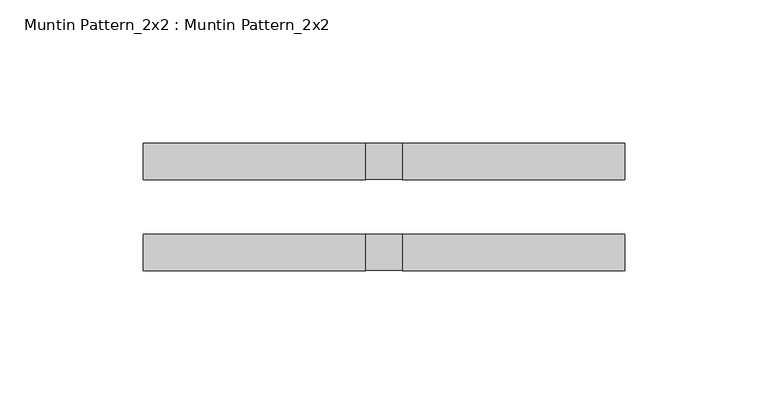
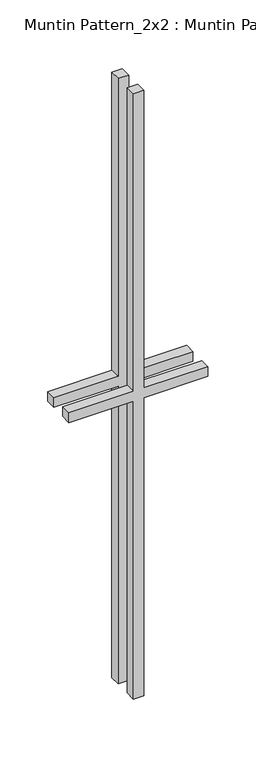
"""IFC4 building model written with IfcOpenShell, lengths in millimetres: proxy geometry, Muntin Pattern_2x2 : Muntin Pattern_2x2."""

from ifc_helpers import new_model, si_unit, frame, origin, place, context, project, spatial, polyline, outline, extrude, source, transform, mapped, element, save


def muntin_pattern_2x2_muntin_pattern_2x2_53152e2c(model_context):
    return source(origin(), model_context, "Body", "SweptSolid", [
        extrude(outline(polyline([(393.7, -6.35), (393.7, -84.1375), (381.0, -84.1375), (381.0, -6.35), (0.0, -6.35), (0.0, 6.35), (381.0, 6.35), (381.0, 84.1375), (393.7, 84.1375), (393.7, 6.35), (774.7, 6.35), (774.7, -6.35), (393.7, -6.35)])), frame((0.0, 9.525, 0.0), z_axis=(0.0, 1.0, 0.0), x_axis=(0.0, 0.0, 1.0)), (0.0, 0.0, 1.0), 12.7),
        extrude(outline(polyline([(393.7, -6.35), (393.7, -84.1375), (381.0, -84.1375), (381.0, -6.35), (0.0, -6.35), (0.0, 6.35), (381.0, 6.35), (381.0, 84.1375), (393.7, 84.1375), (393.7, 6.35), (774.7, 6.35), (774.7, -6.35), (393.7, -6.35)])), frame((0.0, -22.225, 0.0), z_axis=(0.0, 1.0, 0.0), x_axis=(0.0, 0.0, 1.0)), (0.0, 0.0, 1.0), 12.7),
    ])


if __name__ == "__main__":
    model = new_model("IFC4")
    model_context = context("Model", 3, world=origin())
    ifc_project = project(units=[si_unit("LENGTHUNIT", "METRE", prefix="MILLI")], contexts=[model_context])
    site = spatial("IfcSite", under=ifc_project)
    building = spatial("IfcBuilding", under=site)
    placement = place(None, origin())
    muntin_pattern_2x2_muntin_pattern_2x2_shape = muntin_pattern_2x2_muntin_pattern_2x2_53152e2c(model_context)
    element("IfcBuildingElementProxy", 1, Name="Muntin Pattern_2x2 : Muntin Pattern_2x2", ObjectType="Muntin Pattern_2x2 : Muntin Pattern_2x2", at=placement, inside=building, context=model_context, shape_type="MappedRepresentation", body=[
        mapped(muntin_pattern_2x2_muntin_pattern_2x2_shape, transform((0.0, 0.0, 0.0), x_axis=(1.0, 0.0, 0.0), y_axis=(0.0, 1.0, 0.0), z_axis=(0.0, 0.0, 1.0))),
    ])
    save(model, "model.ifc")

# Revit data of these elements
# Type "Muntin Pattern_2x2 : Muntin Pattern_2x2"
#   Width [instance default] = 4' - 0"
#   Thickness = 0' - 0 1/2"
#   Height [instance default] = 4' - 0"
#   Distance = 0' - 0 3/4"
#   Interior Material [instance default] = none
#   Exterior Material [instance default] = none
#   Default Elevation = 0
# Element 1 (IfcBuildingElementProxy, "Muntin Pattern_2x2 : Muntin Pattern_2x2")
#   Width = 0' - 6 5/8"
#   Height = 2' - 6 1/2"
#   Interior Material = Wood - Stained
#   Exterior Material = Clad - White
#   Materials on its faces: "Clad - White", "Wood - Stained"
# Materials
#   "Clad - White": class "Wood", colour RGB 242 242 238, transparency 0, Cost = 0
#   "Wood - Stained": class "Wood", colour RGB 224 178 126, transparency 0, Cost = 0
